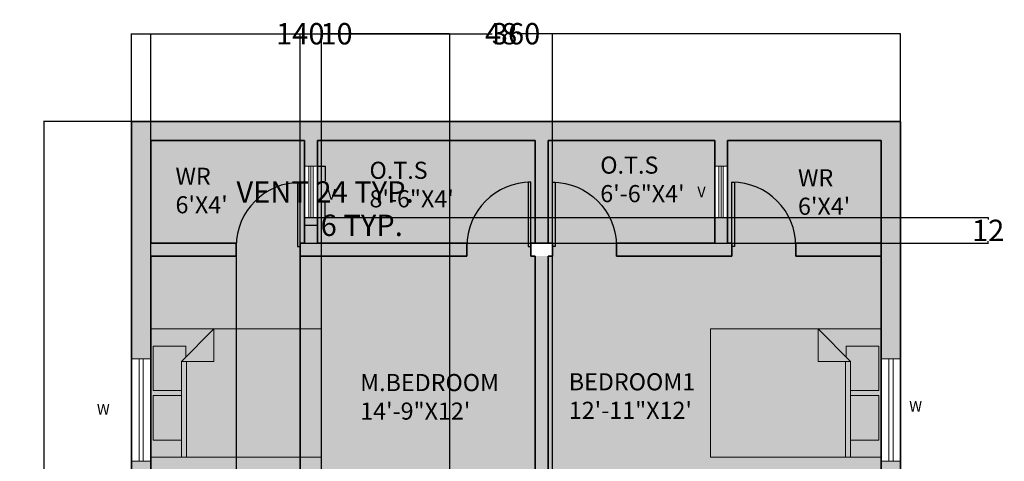
# Model space of a CAD drawing. Units: inches. Extents: x 286 to 756, y 360 to 1175.
# Tile 4 of 4: x 286 to 746, y 969 to 1175. Entities that reach past the tile are written whole.
import ezdxf

# ---------------------------------------------------------------- set-up
doc = ezdxf.new("R2010")
doc.units = ezdxf.units.IN
doc.header["$MEASUREMENT"] = 0
for name, color, linetype, lineweight in [('A-ANNO-DIMS', 2, 'Continuous', 18), ('A-ANNO-TEXT', 7, 'Continuous', 18), ('A-AREA-IDEN', 7, 'Continuous', 18), ('A-GLAZ', 4, 'Continuous', 18), ('A-WALL', 7, 'Continuous', 35), ('DOOR', 6, 'Continuous', 25), ('FUR', 8, 'Continuous', 18)]:
    doc.layers.add(name, color=color, linetype=linetype, lineweight=lineweight)
doc.layers.add('A-FLOR-PATT', color=9, linetype='Continuous', lineweight=13, true_color=0xc7c8ca)
doc.layers.add('A-WALL-PATT', color=18, linetype='Continuous', lineweight=13, true_color=0x000000)
doc.styles.get("Standard").update_dxf_attribs({"font": 'arial.ttf'})
doc.dimstyles.get("Standard").update_dxf_attribs({"dimtxt": 10, "dimasz": 0.18, "dimexe": 0.18, "dimexo": 0.0625, "dimgap": 0.09, "dimtad": 0, "dimtih": 1, "dimtoh": 1, "dimdec": 0, "dimzin": 0, "dimdsep": 46, "dimlunit": 3, "dimtxsty": 'Standard', "dimcen": 0.09, "dimadec": 0, "dimazin": 0, "dimtfac": 1, "dimtdec": 0, "dimtofl": 0, "dimtmove": 0, "dimatfit": 3, "dimfxl": 1, "dimtolj": 1, "dimtzin": 0, "dimarcsym": 0})

# ---------------------------------------------------------------- blocks, each defined once
blk = doc.blocks.new('Bed - Queen')
for p, q in [((0, -80.00003), (0, 0)), ((0, 0), (59.99999, 0)), ((59.99999, 0), (59.99999, -80.00003)), ((7.99999, -1.2), (28.79998, -1.2)), ((7.99999, -14.4), (7.99999, -1.2)), ((28.79998, -1.2), (28.79998, -14.4)), ((31.19999, -1.2), (51.99999, -1.2)), ((31.19999, -14.4), (31.19999, -1.2)), ((51.99999, -1.2), (51.99999, -16.4)), ((0, -14.4), (44.8, -14.4)), ((44.8, -16.8), (0, -16.8)), ((59.99999, -29.6), (44.8, -14.4)), ((44.8, -14.4), (44.8, -29.6)), ((51.99999, -16.4), (46.79936, -16.4)), ((44.8, -29.6), (59.99999, -29.6)), ((59.99999, -80.00003), (0, -80.00003))]:
    blk.add_line(p, q)
blk = doc.blocks.new('*U7')
for p, q in [((0, 0), (0, -6)), ((-40, 0), (-40, -6))]:
    blk.add_line(p, q)
blk.add_lwpolyline([(0, 0), (0, 40), (-1.75, 40), (-1.75, 0)], close=True)
blk.add_arc((0, 0), 40, 90, 180)
blk = doc.blocks.new('*U2')
for p, q in [((0, 0), (0, -6)), ((40, 0), (40, -6))]:
    blk.add_line(p, q)
blk.add_lwpolyline([(0, 0), (0, 40), (1.75, 40), (1.75, 0)], close=True)
blk.add_arc((0, 0), 40, 0, 90)
blk = doc.blocks.new('WIN-48IN-WALL9')
for p, q in [((9, 48), (0, 48)), ((3.5, 0), (3.5, 48)), ((5.5, 0), (5.5, 48)), ((9, 0), (0, 0))]:
    blk.add_line(p, q)
blk = doc.blocks.new('VENT-24IN-WALL6')
for p, q in [((0, 24), (6, 24)), ((2, 0), (2, 24)), ((3, 0), (3, 24)), ((4, 0), (4, 24)), ((0, 0), (6, 0))]:
    blk.add_line(p, q)
blk = doc.blocks.new('*D15')
at = {"layer": 'A-ANNO-DIMS', "color": 0, "lineweight": -2, "transparency": 16777216}
for p, q in [((424.93, 1106.76), (428.65, 1106.76)), ((428.47, 1106.58), (428.47, 1099.87)), ((428.47, 1082.94), (428.47, 1089.64)), ((424.93, 1082.76), (428.65, 1082.76))]:
    blk.add_line(p, q, dxfattribs=at)
at = {"layer": 'A-ANNO-DIMS', "color": 0, "transparency": 16777216}
for points in [[(428.44, 1106.58), (428.5, 1106.58), (428.47, 1106.76)], [(428.44, 1082.94), (428.5, 1082.94), (428.47, 1082.76)]]:
    blk.add_solid(points, dxfattribs=at)
at = {"layer": 'Defpoints', "color": 0, "transparency": 16777216}
for p in [(424.87, 1106.76), (428.47, 1106.76), (424.87, 1082.76)]:
    blk.add_point(p, dxfattribs=at)
at = {"layer": 'A-ANNO-DIMS', "color": 0, "transparency": 16777216, "insert": (428.47, 1094.76), "char_height": 10, "attachment_point": 5}
blk.add_mtext('\\A1;VENT 24 TYP.', dxfattribs=at)
blk = doc.blocks.new('*D16')
at = {"layer": 'A-ANNO-DIMS', "color": 0, "lineweight": -2, "transparency": 16777216}
for p, q in [((418.87, 1082.69), (418.87, 1078.98)), ((419.05, 1079.16), (424.69, 1079.16)), ((424.87, 1082.69), (424.87, 1078.98)), ((424.87, 1079.16), (425.05, 1079.16))]:
    blk.add_line(p, q, dxfattribs=at)
at = {"layer": 'A-ANNO-DIMS', "color": 0, "transparency": 16777216}
for points in [[(419.05, 1079.19), (419.05, 1079.13), (418.87, 1079.16)], [(424.69, 1079.19), (424.69, 1079.13), (424.87, 1079.16)]]:
    blk.add_solid(points, dxfattribs=at)
at = {"layer": 'Defpoints', "color": 0, "transparency": 16777216}
for p in [(418.87, 1082.76), (424.87, 1082.76), (424.87, 1079.16)]:
    blk.add_point(p, dxfattribs=at)
at = {"layer": 'A-ANNO-DIMS', "color": 0, "transparency": 16777216, "insert": (445.62, 1079.16), "char_height": 10, "attachment_point": 5}
blk.add_mtext('\\A1;6 TYP.', dxfattribs=at)
blk = doc.blocks.new('*D19')
at = {"layer": 'A-ANNO-DIMS', "color": 0, "lineweight": -2, "transparency": 16777216}
for p, q in [((337.87, 1127.82), (337.87, 1168.94)), ((338.05, 1168.76), (506.75, 1168.76)), ((697.69, 1168.76), (528.98, 1168.76)), ((697.87, 1127.82), (697.87, 1168.94))]:
    blk.add_line(p, q, dxfattribs=at)
at = {"layer": 'A-ANNO-DIMS', "color": 0, "transparency": 16777216}
for points in [[(338.05, 1168.79), (338.05, 1168.73), (337.87, 1168.76)], [(697.69, 1168.79), (697.69, 1168.73), (697.87, 1168.76)]]:
    blk.add_solid(points, dxfattribs=at)
at = {"layer": 'Defpoints', "color": 0, "transparency": 16777216}
for p in [(697.87, 1168.76), (337.87, 1127.76), (697.87, 1127.76)]:
    blk.add_point(p, dxfattribs=at)
at = {"layer": 'A-ANNO-DIMS', "color": 0, "transparency": 16777216, "insert": (517.87, 1168.76), "char_height": 10, "attachment_point": 5}
blk.add_mtext('\\A1;360', dxfattribs=at)
blk = doc.blocks.new('*D22')
at = {"layer": 'A-ANNO-DIMS', "color": 0, "lineweight": -2, "transparency": 16777216}
for p, q in [((337.8, 1127.76), (296.69, 1127.76)), ((296.87, 1127.58), (296.87, 772.95)), ((296.87, 407.94), (296.87, 762.56)), ((337.8, 407.76), (296.69, 407.76))]:
    blk.add_line(p, q, dxfattribs=at)
at = {"layer": 'A-ANNO-DIMS', "color": 0, "transparency": 16777216}
for points in [[(296.84, 1127.58), (296.9, 1127.58), (296.87, 1127.76)], [(296.84, 407.94), (296.9, 407.94), (296.87, 407.76)]]:
    blk.add_solid(points, dxfattribs=at)
at = {"layer": 'Defpoints', "color": 0, "transparency": 16777216}
for p in [(296.87, 1127.76), (337.87, 1127.76), (337.87, 407.76)]:
    blk.add_point(p, dxfattribs=at)
at = {"layer": 'A-ANNO-DIMS', "color": 0, "transparency": 16777216, "insert": (296.87, 767.76), "char_height": 10, "attachment_point": 5}
blk.add_mtext('\\A1;720', dxfattribs=at)
blk = doc.blocks.new('*D26')
at = {"layer": 'A-ANNO-DIMS', "color": 0, "lineweight": -2, "transparency": 16777216}
for p, q in [((346.87, 656.82), (346.87, 1168.94)), ((347.05, 1168.76), (406.22, 1168.76)), ((486.69, 1168.76), (427.51, 1168.76)), ((486.87, 656.82), (486.87, 1168.94))]:
    blk.add_line(p, q, dxfattribs=at)
at = {"layer": 'A-ANNO-DIMS', "color": 0, "transparency": 16777216}
for points in [[(347.05, 1168.79), (347.05, 1168.73), (346.87, 1168.76)], [(486.69, 1168.79), (486.69, 1168.73), (486.87, 1168.76)]]:
    blk.add_solid(points, dxfattribs=at)
at = {"layer": 'Defpoints', "color": 0, "transparency": 16777216}
for p in [(486.87, 1168.76), (346.87, 656.76), (486.87, 656.76)]:
    blk.add_point(p, dxfattribs=at)
at = {"layer": 'A-ANNO-DIMS', "color": 0, "transparency": 16777216, "insert": (416.87, 1168.76), "char_height": 10, "attachment_point": 5}
blk.add_mtext('\\A1;140', dxfattribs=at)
blk = doc.blocks.new('*D27')
at = {"layer": 'A-ANNO-DIMS', "color": 0, "lineweight": -2, "transparency": 16777216}
for p, q in [((486.87, 656.82), (486.87, 1168.94)), ((487.05, 1168.76), (503.4, 1168.76)), ((534.69, 1168.76), (518.33, 1168.76)), ((534.87, 656.82), (534.87, 1168.94))]:
    blk.add_line(p, q, dxfattribs=at)
at = {"layer": 'A-ANNO-DIMS', "color": 0, "transparency": 16777216}
for points in [[(487.05, 1168.79), (487.05, 1168.73), (486.87, 1168.76)], [(534.69, 1168.79), (534.69, 1168.73), (534.87, 1168.76)]]:
    blk.add_solid(points, dxfattribs=at)
at = {"layer": 'Defpoints', "color": 0, "transparency": 16777216}
for p in [(534.87, 1168.76), (486.87, 656.76), (534.87, 656.76)]:
    blk.add_point(p, dxfattribs=at)
at = {"layer": 'A-ANNO-DIMS', "color": 0, "transparency": 16777216, "insert": (510.87, 1168.76), "char_height": 10, "attachment_point": 5}
blk.add_mtext('\\A1;48', dxfattribs=at)
blk = doc.blocks.new('*D33')
at = {"layer": 'A-ANNO-DIMS', "color": 0, "lineweight": -2, "transparency": 16777216}
for p, q in [((416.87, 452.82), (416.87, 1168.94)), ((417.05, 1168.76), (426.69, 1168.76)), ((426.87, 452.82), (426.87, 1168.94)), ((426.87, 1168.76), (427.05, 1168.76))]:
    blk.add_line(p, q, dxfattribs=at)
at = {"layer": 'A-ANNO-DIMS', "color": 0, "transparency": 16777216}
for points in [[(417.05, 1168.79), (417.05, 1168.73), (416.87, 1168.76)], [(426.69, 1168.79), (426.69, 1168.73), (426.87, 1168.76)]]:
    blk.add_solid(points, dxfattribs=at)
at = {"layer": 'Defpoints', "color": 0, "transparency": 16777216}
for p in [(426.87, 1168.76), (416.87, 452.76), (426.87, 452.76)]:
    blk.add_point(p, dxfattribs=at)
at = {"layer": 'A-ANNO-DIMS', "color": 0, "transparency": 16777216, "insert": (433.81, 1168.76), "char_height": 10, "attachment_point": 5}
blk.add_mtext('\\A1;10', dxfattribs=at)
blk = doc.blocks.new('*D34')
at = {"layer": 'A-ANNO-DIMS', "color": 0, "lineweight": -2, "transparency": 16777216}
for p, q in [((346.87, 1064.69), (346.87, 366.58)), ((386.87, 1064.69), (386.87, 366.58)), ((347.05, 366.76), (359.43, 366.76)), ((386.69, 366.76), (374.3, 366.76))]:
    blk.add_line(p, q, dxfattribs=at)
at = {"layer": 'A-ANNO-DIMS', "color": 0, "transparency": 16777216}
for points in [[(347.05, 366.79), (347.05, 366.73), (346.87, 366.76)], [(386.69, 366.79), (386.69, 366.73), (386.87, 366.76)]]:
    blk.add_solid(points, dxfattribs=at)
at = {"layer": 'Defpoints', "color": 0, "transparency": 16777216}
for p in [(346.87, 1064.76), (386.87, 1064.76), (386.87, 366.76)]:
    blk.add_point(p, dxfattribs=at)
at = {"layer": 'A-ANNO-DIMS', "color": 0, "transparency": 16777216, "insert": (366.87, 366.76), "char_height": 10, "attachment_point": 5}
blk.add_mtext('\\A1;40', dxfattribs=at)
blk = doc.blocks.new('*D35')
at = {"layer": 'A-ANNO-DIMS', "color": 0, "lineweight": -2, "transparency": 16777216}
for p, q in [((386.87, 1064.69), (386.87, 366.58)), ((416.87, 1064.69), (416.87, 366.58)), ((387.05, 366.76), (394.63, 366.76)), ((416.69, 366.76), (409.1, 366.76))]:
    blk.add_line(p, q, dxfattribs=at)
at = {"layer": 'A-ANNO-DIMS', "color": 0, "transparency": 16777216}
for points in [[(387.05, 366.79), (387.05, 366.73), (386.87, 366.76)], [(416.69, 366.79), (416.69, 366.73), (416.87, 366.76)]]:
    blk.add_solid(points, dxfattribs=at)
at = {"layer": 'Defpoints', "color": 0, "transparency": 16777216}
for p in [(386.87, 1064.76), (416.87, 1064.76), (416.87, 366.76)]:
    blk.add_point(p, dxfattribs=at)
at = {"layer": 'A-ANNO-DIMS', "color": 0, "transparency": 16777216, "insert": (401.87, 366.76), "char_height": 10, "attachment_point": 5}
blk.add_mtext('\\A1;30', dxfattribs=at)
blk = doc.blocks.new('*D36')
at = {"layer": 'A-ANNO-DIMS', "color": 0, "lineweight": -2, "transparency": 16777216}
for p, q in [((418.93, 1082.76), (739.05, 1082.76)), ((738.87, 1082.58), (738.87, 1081.87)), ((418.93, 1070.76), (739.05, 1070.76)), ((738.87, 1070.94), (738.87, 1071.65))]:
    blk.add_line(p, q, dxfattribs=at)
at = {"layer": 'A-ANNO-DIMS', "color": 0, "transparency": 16777216}
for points in [[(738.84, 1082.58), (738.9, 1082.58), (738.87, 1082.76)], [(738.84, 1070.94), (738.9, 1070.94), (738.87, 1070.76)]]:
    blk.add_solid(points, dxfattribs=at)
at = {"layer": 'Defpoints', "color": 0, "transparency": 16777216}
for p in [(418.87, 1082.76), (738.87, 1082.76), (418.87, 1070.76)]:
    blk.add_point(p, dxfattribs=at)
at = {"layer": 'A-ANNO-DIMS', "color": 0, "transparency": 16777216, "insert": (738.87, 1076.76), "char_height": 10, "attachment_point": 5}
blk.add_mtext('\\A1;12', dxfattribs=at)

msp = doc.modelspace()

# ---------------------------------------------------------------- hatches: boundary and pattern name
at = {"layer": 'A-FLOR-PATT'}
h = msp.add_hatch(color=256, dxfattribs=at)
h.dxf.hatch_style = 1
h.paths.add_polyline_path([(526.865, 1064.756), (386.892, 1064.756), (346.865, 1064.756), (346.865, 944.756), (448.865, 944.756), (448.865, 920.756), (484.865, 920.756), (484.865, 914.756), (524.865, 914.756), (524.865, 920.756), (526.865, 920.756)])
h.paths.add_polyline_path([(418.865, 1118.756), (346.865, 1118.756), (346.865, 1070.756), (386.865, 1070.756), (386.865, 1064.756), (386.892, 1064.756), (416.865, 1064.756), (416.865, 1070.756), (418.865, 1070.756)])
h.paths.add_polyline_path([(526.865, 1118.756), (424.865, 1118.756), (424.865, 1070.756), (494.865, 1070.756), (494.865, 1064.756), (524.865, 1064.756), (524.865, 1070.756), (526.865, 1070.756)])
h.paths.add_polyline_path([(610.865, 1118.756), (532.865, 1118.756), (532.865, 1070.756), (534.865, 1070.756), (534.865, 1064.756), (564.865, 1064.756), (564.865, 1070.756), (610.865, 1070.756)])
h.paths.add_polyline_path([(688.865, 1118.756), (616.865, 1118.756), (616.865, 1070.756), (618.865, 1070.756), (618.865, 1064.756), (648.865, 1064.756), (648.865, 1070.756), (688.865, 1070.756)])
h.paths.add_polyline_path([(688.865, 1064.756), (648.865, 1064.756), (618.865, 1064.756), (532.865, 1064.756), (532.865, 920.756), (534.865, 920.756), (534.865, 914.756), (570.865, 914.756), (570.865, 920.756), (586.865, 920.756), (586.865, 944.756), (688.865, 944.756)])
h.paths.add_polyline_path([(484.865, 820.756), (478.865, 820.756), (478.865, 844.756), (454.865, 844.756), (454.865, 914.756), (346.865, 914.756), (346.865, 782.756), (478.865, 782.756), (478.865, 784.756), (484.865, 784.756)])
h.paths.add_polyline_path([(688.865, 914.756), (570.865, 914.756), (534.865, 914.756), (484.865, 914.756), (484.865, 820.756), (484.865, 784.756), (484.865, 734.577), (484.865, 662.756), (486.865, 662.756), (486.865, 656.756), (534.865, 656.756), (534.865, 662.756), (688.865, 662.756)])
h.paths.add_polyline_path([(478.865, 734.756), (484.865, 734.756), (484.865, 774.756), (478.865, 774.756), (478.865, 776.756), (388.865, 776.756), (388.865, 734.756), (370.865, 734.756), (370.865, 686.756), (478.865, 686.756)])
h.paths.add_polyline_path([(688.865, 656.756), (534.865, 656.756), (486.865, 656.756), (484.865, 656.756), (346.865, 656.756), (346.865, 536.756), (388.865, 536.756), (388.865, 530.756), (388.865, 506.756), (388.865, 488.756), (388.865, 464.756), (388.865, 452.756), (466.865, 452.756), (466.865, 416.756), (496.865, 416.756), (544.865, 416.756), (580.865, 416.756), (688.865, 416.756)])
h.paths.add_polyline_path([(388.865, 530.756), (346.865, 530.756), (346.865, 494.756), (382.865, 494.756), (382.865, 506.756), (388.865, 506.756)], flags=17)
h.paths.add_polyline_path([(382.865, 464.756), (388.865, 464.756), (388.865, 488.756), (346.865, 488.756), (346.865, 452.756), (382.865, 452.756)], flags=17)
at = {"layer": 'A-WALL-PATT'}
h = msp.add_hatch(color=256, dxfattribs=at)
h.dxf.hatch_style = 1
h.paths.add_polyline_path([(496.865, 416.756), (346.865, 416.756), (346.865, 656.756), (484.865, 656.756), (486.865, 656.756), (486.865, 662.756), (484.865, 662.756), (484.865, 734.577), (478.865, 734.577), (478.865, 662.756), (346.865, 662.756), (346.865, 686.756), (337.865, 686.756), (337.865, 407.756), (496.865, 407.756)])
h.paths.add_polyline_path([(484.865, 784.756), (478.865, 784.756), (478.865, 782.756), (346.865, 782.756), (346.865, 914.756), (406.865, 914.756), (478.865, 914.756), (478.865, 820.756), (484.865, 820.756), (484.865, 920.756), (346.865, 920.756), (346.865, 968.756), (337.865, 968.756), (337.865, 710.756), (346.865, 710.756), (346.865, 734.756), (388.865, 734.756), (388.865, 776.756), (478.865, 776.756), (478.865, 774.756), (484.865, 774.756)])
h.paths.add_polyline_path([(382.865, 776.756), (382.865, 740.756), (346.865, 740.756), (346.865, 776.756)], flags=16)
h.paths.add_polyline_path([(386.865, 1070.756), (346.865, 1070.756), (346.865, 1118.756), (418.865, 1118.756), (418.865, 1106.756), (424.865, 1106.756), (424.865, 1118.756), (526.865, 1118.756), (526.865, 1070.756), (532.865, 1070.756), (532.865, 1118.756), (610.865, 1118.756), (610.865, 1106.756), (616.865, 1106.756), (616.865, 1118.756), (688.865, 1118.756), (688.865, 1016.756), (697.865, 1016.756), (697.865, 1127.756), (337.865, 1127.756), (337.865, 1016.756), (346.865, 1016.756), (346.865, 1030.663), (346.865, 1064.756), (386.865, 1064.756)])
h.paths.add_polyline_path([(494.822, 1069.262, -0.0124335), (494.859, 1070.756), (424.865, 1070.756), (424.865, 1082.756), (418.865, 1082.756), (418.865, 1070.756), (416.865, 1070.756), (416.865, 1069.252), (416.865, 1064.756), (494.822, 1064.756)], flags=17)
h.paths.add_polyline_path([(618.865, 1069.261), (618.865, 1070.756), (616.865, 1070.756), (616.865, 1082.756), (610.865, 1082.756), (610.865, 1070.756), (564.872, 1070.756, -0.0124335), (564.909, 1069.262), (564.909, 1064.756), (618.865, 1064.756)], flags=17)
h.paths.add_polyline_path([(688.865, 1070.756), (648.865, 1070.756), (648.865, 1070.756, -0.0124418), (648.902, 1069.261), (648.902, 1064.756), (688.865, 1064.756)], flags=17)
h.paths.add_polyline_path([(697.865, 968.756), (688.865, 968.756), (688.865, 920.756), (570.865, 920.756), (570.865, 914.756), (688.865, 914.756), (688.865, 873.949), (697.865, 873.949)])
h.paths.add_polyline_path([(697.865, 825.949), (688.865, 825.949), (688.865, 756.879), (697.865, 756.879)])
h.paths.add_polyline_path([(532.865, 1064.756), (526.865, 1064.756), (526.865, 920.756), (524.865, 920.756), (524.865, 914.756), (534.865, 914.756), (534.865, 920.756), (532.865, 920.756)])

# ---------------------------------------------------------------- linework, layer by layer
at = {"layer": 'A-WALL'}
for p, q in [((697.865, 1127.756), (337.865, 1127.756)), ((337.865, 1127.756), (337.865, 407.756)), ((697.865, 407.756), (697.865, 1127.756)), ((346.865, 1118.756), (346.865, 1070.756)), ((418.865, 1118.756), (346.865, 1118.756)), ((418.865, 1118.756), (418.865, 1070.756)), ((418.865, 1070.756), (418.865, 1118.756)), ((424.865, 1118.756), (424.865, 1070.756)), ((526.865, 1118.756), (424.865, 1118.756)), ((526.865, 1118.756), (526.865, 1070.756)), ((532.865, 1118.756), (532.865, 1070.756)), ((610.865, 1118.756), (532.865, 1118.756)), ((610.865, 1070.756), (610.865, 1118.756)), ((688.865, 1118.756), (616.865, 1118.756)), ((616.865, 1070.756), (616.865, 1118.756)), ((688.865, 920.756), (688.865, 1118.756)), ((386.865, 1070.756), (346.865, 1070.756)), ((386.865, 1070.756), (386.865, 1064.756)), ((418.865, 1070.756), (416.865, 1070.756)), ((416.865, 1070.756), (416.865, 1064.756)), ((494.865, 1070.756), (424.865, 1070.756)), ((494.865, 1070.756), (494.865, 1064.756)), ((524.865, 1064.756), (524.865, 1070.756)), ((524.865, 1070.756), (534.865, 1070.756)), ((534.865, 1070.756), (534.865, 1064.756)), ((610.865, 1070.756), (564.865, 1070.756)), ((564.865, 1070.756), (564.865, 1064.756)), ((618.865, 1070.756), (616.865, 1070.756)), ((618.865, 1064.756), (618.865, 1070.756)), ((688.865, 1070.756), (648.865, 1070.756)), ((648.865, 1064.756), (648.865, 1070.756)), ((386.865, 1064.756), (346.865, 1064.756)), ((346.865, 1064.756), (346.865, 920.756)), ((346.865, 920.756), (346.865, 1064.756)), ((416.865, 1064.756), (418.865, 1064.756)), ((494.865, 1064.756), (418.865, 1064.756)), ((526.865, 1064.756), (524.865, 1064.756)), ((526.865, 1064.756), (526.865, 920.756)), ((532.865, 1064.756), (532.865, 920.756)), ((534.865, 1064.756), (532.865, 1064.756)), ((616.865, 1064.756), (564.865, 1064.756)), ((616.865, 1064.756), (618.865, 1064.756)), ((688.865, 1064.756), (648.865, 1064.756))]:
    msp.add_line(p, q, dxfattribs=at)

# ---------------------------------------------------------------- block references
at = {"layer": 'A-GLAZ'}
for name, p in [('VENT-24IN-WALL6', (418.865, 1082.756)), ('WIN-48IN-WALL9', (337.865, 968.756))]:
    msp.add_blockref(name, p, dxfattribs=at)
at = {"layer": 'A-GLAZ', "rotation": 180}
for name, p in [('VENT-24IN-WALL6', (616.865, 1106.756)), ('WIN-48IN-WALL9', (697.865, 1016.756))]:
    msp.add_blockref(name, p, dxfattribs=at)
at = {"layer": 'DOOR'}
for name, p, xscale, yscale, zscale in [('*U7', (416.865, 1069.252), 0.7493264555920812, 0.7493264555920812, 0.7493264555920812), ('*U7', (524.865, 1069.262), 0.7510856449678455, 0.7510856449678455, 0.7510856449678455), ('*U7', (534.865, 1069.262), -0.7510856449678455, 0.7510856449678455, 0.7510856449678455), ('*U2', (618.865, 1069.261), 0.7509296486838268, 0.7509296486838268, 0.7509296486838268)]:
    msp.add_blockref(name, p, dxfattribs=dict(at, xscale=xscale, yscale=yscale, zscale=zscale))
at = {"layer": 'FUR', "rotation": 90}
msp.add_blockref('Bed - Queen', (346.865, 970.663), dxfattribs=at)
at = {"layer": 'FUR', "xscale": -1, "rotation": 270}
msp.add_blockref('Bed - Queen', (688.865, 970.663), dxfattribs=at)

# ---------------------------------------------------------------- texts
at = {"layer": 'A-ANNO-TEXT', "char_height": 5, "attachment_point": 1}
for s, insert in [('V', (602.723, 1097.295)), ('V', (429.456, 1096.134)), ('W', (701.925, 996.961)), ('W', (321.663, 995.579))]:
    msp.add_mtext_dynamic_manual_height_columns(s, width=36.25002, gutter_width=1, heights=[0], dxfattribs=dict(at, insert=insert))
at = {"layer": 'A-AREA-IDEN', "char_height": 8, "attachment_point": 1}
for s, width, insert in [('O.T.S\\P6\'-6"X4\'', 59.48304, (557.294, 1111.304)), ('O.T.S\\P8\'-6"X4\'', 59.48304, (449.255, 1108.875)), ("WR\\P6'X4'", 59.48304, (358.445, 1106.083)), ("WR\\P6'X4'", 59.48304, (649.858, 1105.389)), ('M.BEDROOM\\P14\'-9"X12\'', 65.48511, (444.898, 1009.582)), ('BEDROOM1\\P12\'-11"X12\'', 59.48304, (542.56, 1009.945))]:
    msp.add_mtext_dynamic_manual_height_columns(s, width=width, gutter_width=1, heights=[0], dxfattribs=dict(at, insert=insert))

# ---------------------------------------------------------------- dimensions: what is measured, and where the dimension line sits
at = {"layer": 'A-ANNO-DIMS'}
for base, p1, p2, picture, middle in [((697.865, 1168.756), (337.865, 1127.756), (697.865, 1127.756), '*D19', (517.865, 1168.756)), ((486.865, 1168.756), (346.865, 656.756), (486.865, 656.756), '*D26', (416.865, 1168.756)), ((426.865, 1168.756), (416.865, 452.756), (426.865, 452.756), '*D33', (433.81, 1168.756)), ((534.865, 1168.756), (486.865, 656.756), (534.865, 656.756), '*D27', (510.865, 1168.756)), ((386.865, 366.756), (346.865, 1064.756), (386.865, 1064.756), '*D34', (366.865, 366.756)), ((416.865, 366.756), (386.865, 1064.756), (416.865, 1064.756), '*D35', (401.865, 366.756))]:
    dim = msp.add_linear_dim(base=base, p1=p1, p2=p2, dimstyle='Standard', override={"dimdec": 0, "dimlfac": 1, "dimrnd": 0, "dimzin": 0, "dimdsep": 46, "dimlunit": 2}, dxfattribs=at)
    dim.commit()
    dim.dimension.update_dxf_attribs({"geometry": picture, "text_midpoint": middle})
for base, p1, p2, picture, middle in [((296.865, 1127.756), (337.865, 407.756), (337.865, 1127.756), '*D22', (296.865, 767.756)), ((738.865, 1082.756), (418.865, 1070.756), (418.865, 1082.756), '*D36', (738.865, 1076.756))]:
    dim = msp.add_linear_dim(base=base, p1=p1, p2=p2, angle=90, dimstyle='Standard', override={"dimdec": 0, "dimlfac": 1, "dimrnd": 0, "dimzin": 0, "dimdsep": 46, "dimlunit": 2}, dxfattribs=at)
    dim.commit()
    dim.dimension.update_dxf_attribs({"geometry": picture, "text_midpoint": middle})
dim = msp.add_linear_dim(base=(428.465, 1106.756), p1=(424.865, 1082.756), p2=(424.865, 1106.756), angle=90, text='VENT <> TYP.', dimstyle='Standard', override={"dimdec": 0, "dimlfac": 1, "dimrnd": 0, "dimzin": 0, "dimdsep": 46, "dimlunit": 2}, dxfattribs=at)
dim.commit()
dim.dimension.update_dxf_attribs({"geometry": '*D15', "text_midpoint": (428.465, 1094.756)})
dim = msp.add_linear_dim(base=(424.865, 1079.156), p1=(418.865, 1082.756), p2=(424.865, 1082.756), text='<> TYP.', dimstyle='Standard', override={"dimdec": 0, "dimlfac": 1, "dimrnd": 0, "dimzin": 0, "dimdsep": 46, "dimlunit": 2}, dxfattribs=at)
dim.commit()
dim.dimension.update_dxf_attribs({"geometry": '*D16', "text_midpoint": (445.616, 1079.156)})

doc.saveas('drawing.dxf')
